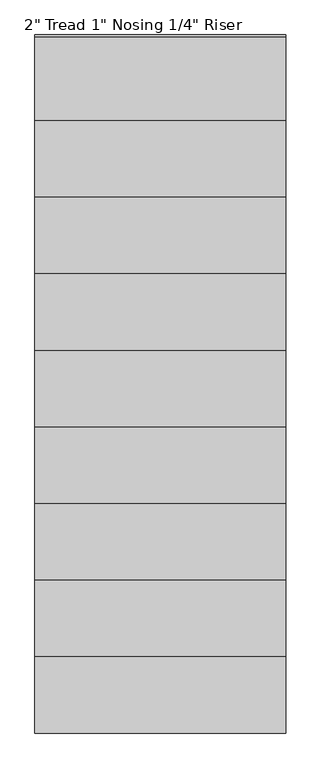
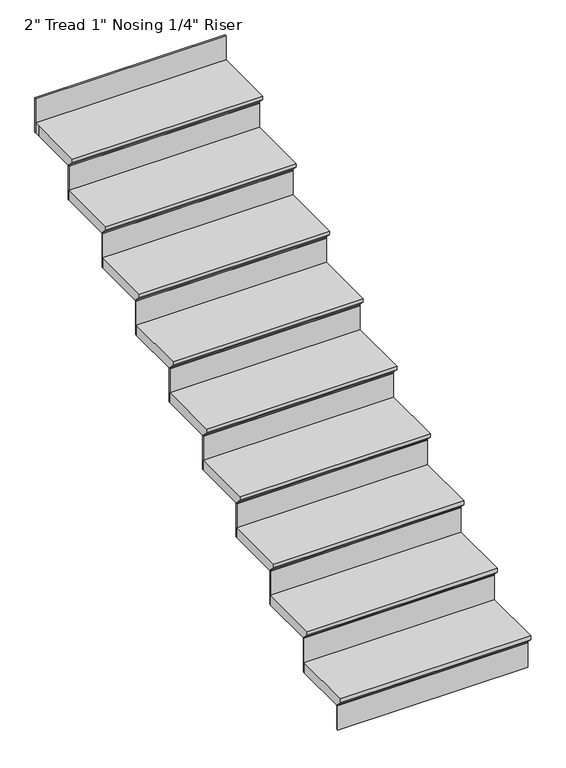
"""IFC4 building model written with IfcOpenShell, lengths in millimetres: stair flight geometry."""

from ifc_helpers import new_model, si_unit, origin, place, context, project, spatial, faceted_brep, source, transform, mapped, element, save


def stair_flight_ed17b8c2(model_context):
    return source(origin(), model_context, "Body", "Brep", [
        faceted_brep([(8378.8260838, -1689.0339187, 154.1318182), (8378.8260838, -1689.0339187, 173.1818182), (7464.4260838, -1689.0339187, 173.1818182), (7464.4260838, -1689.0339187, 154.1318182), (8378.8260838, -1663.6339187, 128.7318182), (7464.4260838, -1663.6339187, 128.7318182), (8378.8260838, -1384.2339187, 173.1818182), (7464.4260838, -1384.2339187, 173.1818182), (7464.4260838, -1663.6339187, 122.3818182), (7464.4260838, -1384.2339187, 122.3818182), (8378.8260838, -1384.2339187, 122.3818182), (8378.8260838, -1663.6339187, 122.3818182)], [[[0, 1, 2, 3]], [[4, 0, 3, 5]], [[2, 1, 6, 7]], [[8, 9, 10, 11]], [[2, 7, 9, 8, 5, 3]], [[8, 11, 4, 5]], [[6, 1, 0, 4, 11, 10]], [[7, 6, 10, 9]]]),
        faceted_brep([(8378.8260838, -1663.6339187, 122.3818182), (8378.8260838, -1663.6339187, 0.0), (8378.8260838, -1657.2839187, 0.0), (8378.8260838, -1657.2839187, 122.3818182), (7464.4260838, -1663.6339187, 122.3818182), (7464.4260838, -1657.2839187, 122.3818182), (7464.4260838, -1657.2839187, 0.0), (7464.4260838, -1663.6339187, 0.0)], [[[0, 1, 2, 3]], [[4, 5, 6, 7]], [[1, 0, 4, 7]], [[2, 1, 7, 6]], [[3, 2, 6, 5]], [[0, 3, 5, 4]]]),
        faceted_brep([(8378.8260838, -1384.2339187, 295.5636364), (8378.8260838, -1384.2339187, 122.3818182), (8378.8260838, -1377.8839187, 122.3818182), (8378.8260838, -1377.8839187, 295.5636364), (7464.4260838, -1384.2339187, 295.5636364), (7464.4260838, -1377.8839187, 295.5636364), (7464.4260838, -1377.8839187, 122.3818182), (7464.4260838, -1384.2339187, 122.3818182)], [[[0, 1, 2, 3]], [[4, 5, 6, 7]], [[1, 0, 4, 7]], [[2, 1, 7, 6]], [[3, 2, 6, 5]], [[0, 3, 5, 4]]]),
        faceted_brep([(7464.4260838, -1409.6339187, 346.3636364), (8378.8260838, -1409.6339187, 346.3636364), (8378.8260838, -1104.8339187, 346.3636364), (7464.4260838, -1104.8339187, 346.3636364), (7464.4260838, -1384.2339187, 295.5636364), (7464.4260838, -1104.8339187, 295.5636364), (8378.8260838, -1104.8339187, 295.5636364), (8378.8260838, -1384.2339187, 295.5636364), (7464.4260838, -1384.2339187, 301.9136364), (7464.4260838, -1409.6339187, 327.3136364), (8378.8260838, -1384.2339187, 301.9136364), (8378.8260838, -1409.6339187, 327.3136364)], [[[0, 1, 2, 3]], [[4, 5, 6, 7]], [[0, 3, 5, 4, 8, 9]], [[4, 7, 10, 8]], [[2, 1, 11, 10, 7, 6]], [[3, 2, 6, 5]], [[11, 1, 0, 9]], [[10, 11, 9, 8]]]),
        faceted_brep([(8378.8260838, -1104.8339187, 468.7454545), (8378.8260838, -1104.8339187, 295.5636364), (8378.8260838, -1098.4839187, 295.5636364), (8378.8260838, -1098.4839187, 468.7454545), (7464.4260838, -1104.8339187, 468.7454545), (7464.4260838, -1098.4839187, 468.7454545), (7464.4260838, -1098.4839187, 295.5636364), (7464.4260838, -1104.8339187, 295.5636364)], [[[0, 1, 2, 3]], [[4, 5, 6, 7]], [[1, 0, 4, 7]], [[2, 1, 7, 6]], [[3, 2, 6, 5]], [[0, 3, 5, 4]]]),
        faceted_brep([(7464.4260838, -1130.2339187, 519.5454545), (8378.8260838, -1130.2339187, 519.5454545), (8378.8260838, -825.4339187, 519.5454545), (7464.4260838, -825.4339187, 519.5454545), (7464.4260838, -1104.8339187, 468.7454545), (7464.4260838, -825.4339187, 468.7454545), (8378.8260838, -825.4339187, 468.7454545), (8378.8260838, -1104.8339187, 468.7454545), (7464.4260838, -1104.8339187, 475.0954545), (7464.4260838, -1130.2339187, 500.4954545), (8378.8260838, -1104.8339187, 475.0954545), (8378.8260838, -1130.2339187, 500.4954545)], [[[0, 1, 2, 3]], [[4, 5, 6, 7]], [[0, 3, 5, 4, 8, 9]], [[4, 7, 10, 8]], [[2, 1, 11, 10, 7, 6]], [[3, 2, 6, 5]], [[11, 1, 0, 9]], [[10, 11, 9, 8]]]),
        faceted_brep([(8378.8260838, -825.4339187, 641.9272727), (8378.8260838, -825.4339187, 468.7454545), (8378.8260838, -819.0839187, 468.7454545), (8378.8260838, -819.0839187, 641.9272727), (7464.4260838, -825.4339187, 641.9272727), (7464.4260838, -819.0839187, 641.9272727), (7464.4260838, -819.0839187, 468.7454545), (7464.4260838, -825.4339187, 468.7454545)], [[[0, 1, 2, 3]], [[4, 5, 6, 7]], [[1, 0, 4, 7]], [[2, 1, 7, 6]], [[3, 2, 6, 5]], [[0, 3, 5, 4]]]),
        faceted_brep([(7464.4260838, -850.8339187, 692.7272727), (8378.8260838, -850.8339187, 692.7272727), (8378.8260838, -546.0339187, 692.7272727), (7464.4260838, -546.0339187, 692.7272727), (7464.4260838, -825.4339187, 641.9272727), (7464.4260838, -546.0339187, 641.9272727), (8378.8260838, -546.0339187, 641.9272727), (8378.8260838, -825.4339187, 641.9272727), (7464.4260838, -825.4339187, 648.2772727), (7464.4260838, -850.8339187, 673.6772727), (8378.8260838, -825.4339187, 648.2772727), (8378.8260838, -850.8339187, 673.6772727)], [[[0, 1, 2, 3]], [[4, 5, 6, 7]], [[0, 3, 5, 4, 8, 9]], [[4, 7, 10, 8]], [[2, 1, 11, 10, 7, 6]], [[3, 2, 6, 5]], [[11, 1, 0, 9]], [[10, 11, 9, 8]]]),
        faceted_brep([(8378.8260838, -546.0339187, 815.1090909), (8378.8260838, -546.0339187, 641.9272727), (8378.8260838, -539.6839187, 641.9272727), (8378.8260838, -539.6839187, 815.1090909), (7464.4260838, -546.0339187, 815.1090909), (7464.4260838, -539.6839187, 815.1090909), (7464.4260838, -539.6839187, 641.9272727), (7464.4260838, -546.0339187, 641.9272727)], [[[0, 1, 2, 3]], [[4, 5, 6, 7]], [[1, 0, 4, 7]], [[2, 1, 7, 6]], [[3, 2, 6, 5]], [[0, 3, 5, 4]]]),
        faceted_brep([(7464.4260838, -571.4339187, 865.9090909), (8378.8260838, -571.4339187, 865.9090909), (8378.8260838, -266.6339187, 865.9090909), (7464.4260838, -266.6339187, 865.9090909), (7464.4260838, -546.0339187, 815.1090909), (7464.4260838, -266.6339187, 815.1090909), (8378.8260838, -266.6339187, 815.1090909), (8378.8260838, -546.0339187, 815.1090909), (7464.4260838, -546.0339187, 821.4590909), (7464.4260838, -571.4339187, 846.8590909), (8378.8260838, -546.0339187, 821.4590909), (8378.8260838, -571.4339187, 846.8590909)], [[[0, 1, 2, 3]], [[4, 5, 6, 7]], [[0, 3, 5, 4, 8, 9]], [[4, 7, 10, 8]], [[2, 1, 11, 10, 7, 6]], [[3, 2, 6, 5]], [[11, 1, 0, 9]], [[10, 11, 9, 8]]]),
        faceted_brep([(8378.8260838, -266.6339187, 988.2909091), (8378.8260838, -266.6339187, 815.1090909), (8378.8260838, -260.2839187, 815.1090909), (8378.8260838, -260.2839187, 988.2909091), (7464.4260838, -266.6339187, 988.2909091), (7464.4260838, -260.2839187, 988.2909091), (7464.4260838, -260.2839187, 815.1090909), (7464.4260838, -266.6339187, 815.1090909)], [[[0, 1, 2, 3]], [[4, 5, 6, 7]], [[1, 0, 4, 7]], [[2, 1, 7, 6]], [[3, 2, 6, 5]], [[0, 3, 5, 4]]]),
        faceted_brep([(7464.4260838, -292.0339187, 1039.0909091), (8378.8260838, -292.0339187, 1039.0909091), (8378.8260838, 12.7660813, 1039.0909091), (7464.4260838, 12.7660813, 1039.0909091), (7464.4260838, -266.6339187, 988.2909091), (7464.4260838, 12.7660813, 988.2909091), (8378.8260838, 12.7660813, 988.2909091), (8378.8260838, -266.6339187, 988.2909091), (7464.4260838, -266.6339187, 994.6409091), (7464.4260838, -292.0339187, 1020.0409091), (8378.8260838, -266.6339187, 994.6409091), (8378.8260838, -292.0339187, 1020.0409091)], [[[0, 1, 2, 3]], [[4, 5, 6, 7]], [[0, 3, 5, 4, 8, 9]], [[4, 7, 10, 8]], [[2, 1, 11, 10, 7, 6]], [[3, 2, 6, 5]], [[11, 1, 0, 9]], [[10, 11, 9, 8]]]),
        faceted_brep([(8378.8260838, 12.7660813, 1161.4727273), (8378.8260838, 12.7660813, 988.2909091), (8378.8260838, 19.1160813, 988.2909091), (8378.8260838, 19.1160813, 1161.4727273), (7464.4260838, 12.7660813, 1161.4727273), (7464.4260838, 19.1160813, 1161.4727273), (7464.4260838, 19.1160813, 988.2909091), (7464.4260838, 12.7660813, 988.2909091)], [[[0, 1, 2, 3]], [[4, 5, 6, 7]], [[1, 0, 4, 7]], [[2, 1, 7, 6]], [[3, 2, 6, 5]], [[0, 3, 5, 4]]]),
        faceted_brep([(7464.4260838, -12.6339187, 1212.2727273), (8378.8260838, -12.6339187, 1212.2727273), (8378.8260838, 292.1660813, 1212.2727273), (7464.4260838, 292.1660813, 1212.2727273), (7464.4260838, 12.7660813, 1161.4727273), (7464.4260838, 292.1660813, 1161.4727273), (8378.8260838, 292.1660813, 1161.4727273), (8378.8260838, 12.7660813, 1161.4727273), (7464.4260838, 12.7660813, 1167.8227273), (7464.4260838, -12.6339187, 1193.2227273), (8378.8260838, 12.7660813, 1167.8227273), (8378.8260838, -12.6339187, 1193.2227273)], [[[0, 1, 2, 3]], [[4, 5, 6, 7]], [[0, 3, 5, 4, 8, 9]], [[4, 7, 10, 8]], [[2, 1, 11, 10, 7, 6]], [[3, 2, 6, 5]], [[11, 1, 0, 9]], [[10, 11, 9, 8]]]),
        faceted_brep([(8378.8260838, 292.1660813, 1334.6545455), (8378.8260838, 292.1660813, 1161.4727273), (8378.8260838, 298.5160813, 1161.4727273), (8378.8260838, 298.5160813, 1334.6545455), (7464.4260838, 292.1660813, 1334.6545455), (7464.4260838, 298.5160813, 1334.6545455), (7464.4260838, 298.5160813, 1161.4727273), (7464.4260838, 292.1660813, 1161.4727273)], [[[0, 1, 2, 3]], [[4, 5, 6, 7]], [[1, 0, 4, 7]], [[2, 1, 7, 6]], [[3, 2, 6, 5]], [[0, 3, 5, 4]]]),
        faceted_brep([(7464.4260838, 266.7660813, 1385.4545455), (8378.8260838, 266.7660813, 1385.4545455), (8378.8260838, 571.5660813, 1385.4545455), (7464.4260838, 571.5660813, 1385.4545455), (7464.4260838, 292.1660813, 1334.6545455), (7464.4260838, 571.5660813, 1334.6545455), (8378.8260838, 571.5660813, 1334.6545455), (8378.8260838, 292.1660813, 1334.6545455), (7464.4260838, 292.1660813, 1341.0045455), (7464.4260838, 266.7660813, 1366.4045455), (8378.8260838, 292.1660813, 1341.0045455), (8378.8260838, 266.7660813, 1366.4045455)], [[[0, 1, 2, 3]], [[4, 5, 6, 7]], [[0, 3, 5, 4, 8, 9]], [[4, 7, 10, 8]], [[2, 1, 11, 10, 7, 6]], [[3, 2, 6, 5]], [[11, 1, 0, 9]], [[10, 11, 9, 8]]]),
        faceted_brep([(8378.8260838, 850.9660813, 1681.0181818), (8378.8260838, 850.9660813, 1507.8363636), (8378.8260838, 857.3160813, 1507.8363636), (8378.8260838, 857.3160813, 1681.0181818), (7464.4260838, 850.9660813, 1681.0181818), (7464.4260838, 857.3160813, 1681.0181818), (7464.4260838, 857.3160813, 1507.8363636), (7464.4260838, 850.9660813, 1507.8363636)], [[[0, 1, 2, 3]], [[4, 5, 6, 7]], [[1, 0, 4, 7]], [[2, 1, 7, 6]], [[3, 2, 6, 5]], [[0, 3, 5, 4]]]),
        faceted_brep([(8378.8260838, 571.5660813, 1507.8363636), (8378.8260838, 571.5660813, 1334.6545455), (8378.8260838, 577.9160813, 1334.6545455), (8378.8260838, 577.9160813, 1507.8363636), (7464.4260838, 571.5660813, 1507.8363636), (7464.4260838, 577.9160813, 1507.8363636), (7464.4260838, 577.9160813, 1334.6545455), (7464.4260838, 571.5660813, 1334.6545455)], [[[0, 1, 2, 3]], [[4, 5, 6, 7]], [[1, 0, 4, 7]], [[2, 1, 7, 6]], [[3, 2, 6, 5]], [[0, 3, 5, 4]]]),
        faceted_brep([(7464.4260838, 850.9660813, 1558.6363636), (7464.4260838, 825.5660813, 1558.6363636), (7464.4260838, 546.1660813, 1558.6363636), (8378.8260838, 546.1660813, 1558.6363636), (8378.8260838, 850.9660813, 1558.6363636), (7464.4260838, 825.5660813, 1507.8363636), (7464.4260838, 850.9660813, 1507.8363636), (8378.8260838, 850.9660813, 1507.8363636), (8378.8260838, 571.5660813, 1507.8363636), (7464.4260838, 571.5660813, 1507.8363636), (7464.4260838, 571.5660813, 1514.1863636), (7464.4260838, 546.1660813, 1539.5863636), (8378.8260838, 571.5660813, 1514.1863636), (8378.8260838, 546.1660813, 1539.5863636)], [[[0, 1, 2, 3, 4]], [[5, 6, 7, 8, 9]], [[1, 0, 6, 5]], [[2, 1, 5, 9, 10, 11]], [[9, 8, 12, 10]], [[4, 3, 13, 12, 8, 7]], [[0, 4, 7, 6]], [[13, 3, 2, 11]], [[12, 13, 11, 10]]]),
    ])


if __name__ == "__main__":
    model = new_model("IFC4")
    model_context = context("Model", 3, world=origin())
    ifc_project = project(units=[si_unit("LENGTHUNIT", "METRE", prefix="MILLI")], contexts=[model_context])
    site = spatial("IfcSite", under=ifc_project)
    building = spatial("IfcBuilding", under=site)
    placement = place(None, origin())
    stair_flight_shape = stair_flight_ed17b8c2(model_context)
    element("IfcStairFlight", 1, ObjectType="2\" Tread 1\" Nosing 1/4\" Riser", at=placement, inside=building, context=model_context, shape_type="MappedRepresentation", body=[
        mapped(stair_flight_shape, transform((0.0, 0.0, 0.0), x_axis=(1.0, 0.0, 0.0), y_axis=(0.0, 1.0, 0.0), z_axis=(0.0, 0.0, 1.0))),
    ])
    save(model, "model.ifc")
